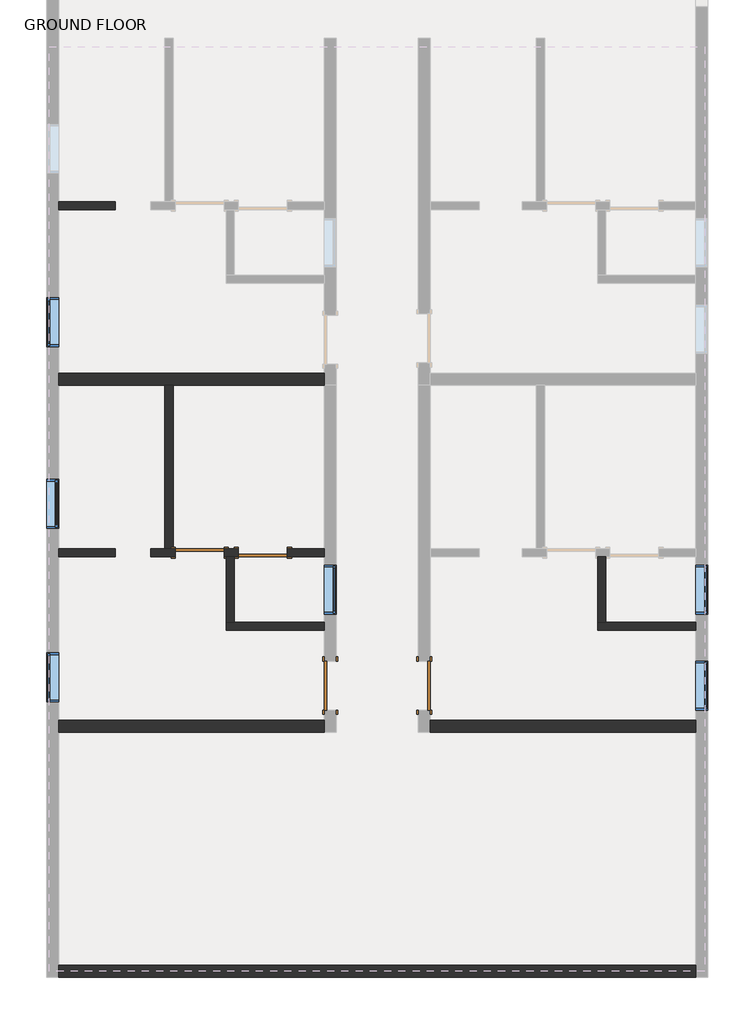
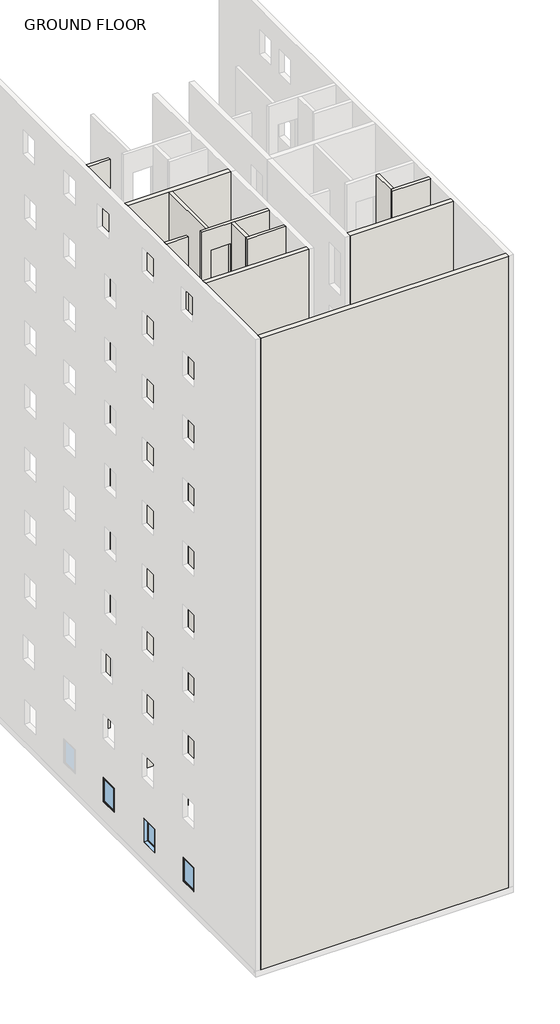
# One storey, part 1 of 7: 12 walls, 6 windows, 4 doors.
"""IFC4 building model written with IfcOpenShell, lengths in millimetres."""

from ifc_helpers import new_model, si_unit, origin, origin_with_axes, place, context, project, spatial, polyline, outline, extrude, faceted_brep, transform, mapped, element, save
from components import door_686f89d2, door_16372e1c, door_a90ba1ad, door_0ca8825f, window_c1f32544

model = new_model("IFC4")

# Units and contexts
model_context = context("Model", 3, world=origin())
ifc_project = project(units=[si_unit("LENGTHUNIT", "METRE", prefix="MILLI")], contexts=[model_context])

# Site, building, storey
site = spatial("IfcSite", under=ifc_project)
building = spatial("IfcBuilding", under=site)
storey = spatial("IfcBuildingStorey", under=building, Name="GROUND FLOOR", Elevation=0.0)

# Doors
placement = place(None, origin())
door_shape = door_686f89d2(model_context)
element("IfcDoor", 1, ObjectType="Single-Flush : 36\" x 84\"", at=placement, inside=storey, context=model_context, shape_type="MappedRepresentation", body=[
    mapped(door_shape, transform((-9863.5902461, -7478.7289408, 0.0), x_axis=(-1.0, 0.0, 0.0), y_axis=(0.0, -1.0, 0.0), z_axis=(0.0, 0.0, 1.0))),
])
door_2_shape = door_16372e1c(model_context)
element("IfcDoor", 2, ObjectType="Single-Flush : 36\" x 84\"", at=placement, inside=storey, context=model_context, shape_type="MappedRepresentation", body=[
    mapped(door_2_shape, transform((-8682.4902461, -7478.7289408, 0.0), x_axis=(-1.0, 0.0, 0.0), y_axis=(0.0, -1.0, 0.0), z_axis=(0.0, 0.0, 1.0))),
])
door_3_shape = door_a90ba1ad(model_context)
element("IfcDoor", 3, ObjectType="Single-Flush : 36\" x 84\"", at=placement, inside=storey, context=model_context, shape_type="MappedRepresentation", body=[
    mapped(door_3_shape, transform((-7425.1902461, -9955.2289408, 0.0), x_axis=(0.0, -1.0, 0.0), y_axis=(1.0, 0.0, 0.0), z_axis=(0.0, 0.0, 1.0))),
])
door_4_shape = door_0ca8825f(model_context)
element("IfcDoor", 4, ObjectType="Single-Flush : 36\" x 84\"", at=placement, inside=storey, context=model_context, shape_type="MappedRepresentation", body=[
    mapped(door_4_shape, transform((-5672.5902461, -9955.2289408, 0.0), x_axis=(0.0, -1.0, 0.0), y_axis=(1.0, 0.0, 0.0), z_axis=(0.0, 0.0, 1.0))),
])

# Walls
element("IfcWall", 5, ObjectType="INNER WALL 2", at=placement, inside=storey, context=model_context, shape_type="Brep", body=[
    faceted_brep([(-605.2902461, -8774.1289408, 0.0), (-2281.6902461, -8774.1289408, 0.0), (-2434.0902461, -8774.1289408, 0.0), (-2434.0902461, -8774.1289408, 32004.0), (-2281.6902461, -8774.1289408, 32004.0), (-605.2902461, -8774.1289408, 32004.0), (-605.2902461, -8926.5289408, 0.0), (-605.2902461, -8926.5289408, 32004.0), (-2434.0902461, -8926.5289408, 32004.0), (-2434.0902461, -8926.5289408, 0.0)], [[[0, 1, 2, 3, 4, 5]], [[6, 7, 8, 9]], [[2, 1, 0, 6, 9]], [[5, 4, 3, 8, 7]], [[3, 2, 9, 8]], [[0, 5, 7, 6]]]),
])
element("IfcWall", 6, ObjectType="INNER WALL 2", at=placement, inside=storey, context=model_context, shape_type="SweptSolid", body=[
    extrude(outline(polyline([(-2281.6902461, -7554.9289408), (-2281.6902461, -8774.1289408), (-2434.0902461, -8774.1289408), (-2434.0902461, -7554.9289408), (-2281.6902461, -7554.9289408)])), origin_with_axes(), (0.0, 0.0, 1.0), 32004.0),
])
element("IfcWall", 7, ObjectType="INNER WALL 2", at=placement, inside=storey, context=model_context, shape_type="Brep", body=[
    faceted_brep([(-9406.3902461, -7554.9289408, 0.0), (-9368.2902461, -7554.9289408, 0.0), (-9215.8902461, -7554.9289408, 0.0), (-9139.6902461, -7554.9289408, 0.0), (-9139.6902461, -7554.9289408, 2133.6), (-8225.2902461, -7554.9289408, 2133.6), (-8225.2902461, -7554.9289408, 0.0), (-7539.4902461, -7554.9289408, 0.0), (-7539.4902461, -7554.9289408, 32004.0), (-9215.8902461, -7554.9289408, 32004.0), (-9368.2902461, -7554.9289408, 32004.0), (-10777.9902461, -7554.9289408, 32004.0), (-10777.9902461, -7554.9289408, 0.0), (-10320.7902461, -7554.9289408, 0.0), (-10320.7902461, -7554.9289408, 2133.6), (-9406.3902461, -7554.9289408, 2133.6), (-9406.3902461, -7554.9289408, 3200.4), (-10320.7902461, -7554.9289408, 3200.4), (-10320.7902461, -7554.9289408, 5334.0), (-9406.3902461, -7554.9289408, 5334.0), (-8225.2902461, -7554.9289408, 3200.4), (-9139.6902461, -7554.9289408, 3200.4), (-9139.6902461, -7554.9289408, 5334.0), (-8225.2902461, -7554.9289408, 5334.0), (-9406.3902461, -7554.9289408, 6400.8), (-10320.7902461, -7554.9289408, 6400.8), (-10320.7902461, -7554.9289408, 8534.4), (-9406.3902461, -7554.9289408, 8534.4), (-8225.2902461, -7554.9289408, 6400.8), (-9139.6902461, -7554.9289408, 6400.8), (-9139.6902461, -7554.9289408, 8534.4), (-8225.2902461, -7554.9289408, 8534.4), (-9406.3902461, -7554.9289408, 9601.2), (-10320.7902461, -7554.9289408, 9601.2), (-10320.7902461, -7554.9289408, 11734.8), (-9406.3902461, -7554.9289408, 11734.8), (-8225.2902461, -7554.9289408, 9601.2), (-9139.6902461, -7554.9289408, 9601.2), (-9139.6902461, -7554.9289408, 11734.8), (-8225.2902461, -7554.9289408, 11734.8), (-9406.3902461, -7554.9289408, 12801.6), (-10320.7902461, -7554.9289408, 12801.6), (-10320.7902461, -7554.9289408, 14935.2), (-9406.3902461, -7554.9289408, 14935.2), (-8225.2902461, -7554.9289408, 12801.6), (-9139.6902461, -7554.9289408, 12801.6), (-9139.6902461, -7554.9289408, 14935.2), (-8225.2902461, -7554.9289408, 14935.2), (-9406.3902461, -7554.9289408, 16002.0), (-10320.7902461, -7554.9289408, 16002.0), (-10320.7902461, -7554.9289408, 18135.6), (-9406.3902461, -7554.9289408, 18135.6), (-8225.2902461, -7554.9289408, 16002.0), (-9139.6902461, -7554.9289408, 16002.0), (-9139.6902461, -7554.9289408, 18135.6), (-8225.2902461, -7554.9289408, 18135.6), (-9406.3902461, -7554.9289408, 19202.4), (-10320.7902461, -7554.9289408, 19202.4), (-10320.7902461, -7554.9289408, 21336.0), (-9406.3902461, -7554.9289408, 21336.0), (-8225.2902461, -7554.9289408, 19202.4), (-9139.6902461, -7554.9289408, 19202.4), (-9139.6902461, -7554.9289408, 21336.0), (-8225.2902461, -7554.9289408, 21336.0), (-9406.3902461, -7554.9289408, 22402.8), (-10320.7902461, -7554.9289408, 22402.8), (-10320.7902461, -7554.9289408, 24536.4), (-9406.3902461, -7554.9289408, 24536.4), (-8225.2902461, -7554.9289408, 22402.8), (-9139.6902461, -7554.9289408, 22402.8), (-9139.6902461, -7554.9289408, 24536.4), (-8225.2902461, -7554.9289408, 24536.4), (-9406.3902461, -7554.9289408, 25603.2), (-10320.7902461, -7554.9289408, 25603.2), (-10320.7902461, -7554.9289408, 27736.8), (-9406.3902461, -7554.9289408, 27736.8), (-8225.2902461, -7554.9289408, 25603.2), (-9139.6902461, -7554.9289408, 25603.2), (-9139.6902461, -7554.9289408, 27736.8), (-8225.2902461, -7554.9289408, 27736.8), (-9406.3902461, -7554.9289408, 28803.6), (-10320.7902461, -7554.9289408, 28803.6), (-10320.7902461, -7554.9289408, 30937.2), (-9406.3902461, -7554.9289408, 30937.2), (-8225.2902461, -7554.9289408, 28803.6), (-9139.6902461, -7554.9289408, 28803.6), (-9139.6902461, -7554.9289408, 30937.2), (-8225.2902461, -7554.9289408, 30937.2), (-9139.6902461, -7402.5289408, 2133.6), (-9139.6902461, -7402.5289408, 0.0), (-9406.3902461, -7402.5289408, 0.0), (-9406.3902461, -7402.5289408, 2133.6), (-10320.7902461, -7402.5289408, 2133.6), (-10320.7902461, -7402.5289408, 0.0), (-10358.8902461, -7402.5289408, 0.0), (-10511.2902461, -7402.5289408, 0.0), (-10777.9902461, -7402.5289408, 0.0), (-10777.9902461, -7402.5289408, 32004.0), (-10511.2902461, -7402.5289408, 32004.0), (-10358.8902461, -7402.5289408, 32004.0), (-7539.4902461, -7402.5289408, 32004.0), (-7539.4902461, -7402.5289408, 0.0), (-8225.2902461, -7402.5289408, 0.0), (-8225.2902461, -7402.5289408, 2133.6), (-9406.3902461, -7402.5289408, 3200.4), (-9406.3902461, -7402.5289408, 5334.0), (-10320.7902461, -7402.5289408, 5334.0), (-10320.7902461, -7402.5289408, 3200.4), (-8225.2902461, -7402.5289408, 3200.4), (-8225.2902461, -7402.5289408, 5334.0), (-9139.6902461, -7402.5289408, 5334.0), (-9139.6902461, -7402.5289408, 3200.4), (-9406.3902461, -7402.5289408, 6400.8), (-9406.3902461, -7402.5289408, 8534.4), (-10320.7902461, -7402.5289408, 8534.4), (-10320.7902461, -7402.5289408, 6400.8), (-8225.2902461, -7402.5289408, 6400.8), (-8225.2902461, -7402.5289408, 8534.4), (-9139.6902461, -7402.5289408, 8534.4), (-9139.6902461, -7402.5289408, 6400.8), (-9406.3902461, -7402.5289408, 9601.2), (-9406.3902461, -7402.5289408, 11734.8), (-10320.7902461, -7402.5289408, 11734.8), (-10320.7902461, -7402.5289408, 9601.2), (-8225.2902461, -7402.5289408, 9601.2), (-8225.2902461, -7402.5289408, 11734.8), (-9139.6902461, -7402.5289408, 11734.8), (-9139.6902461, -7402.5289408, 9601.2), (-9406.3902461, -7402.5289408, 12801.6), (-9406.3902461, -7402.5289408, 14935.2), (-10320.7902461, -7402.5289408, 14935.2), (-10320.7902461, -7402.5289408, 12801.6), (-8225.2902461, -7402.5289408, 12801.6), (-8225.2902461, -7402.5289408, 14935.2), (-9139.6902461, -7402.5289408, 14935.2), (-9139.6902461, -7402.5289408, 12801.6), (-9406.3902461, -7402.5289408, 16002.0), (-9406.3902461, -7402.5289408, 18135.6), (-10320.7902461, -7402.5289408, 18135.6), (-10320.7902461, -7402.5289408, 16002.0), (-8225.2902461, -7402.5289408, 16002.0), (-8225.2902461, -7402.5289408, 18135.6), (-9139.6902461, -7402.5289408, 18135.6), (-9139.6902461, -7402.5289408, 16002.0), (-9406.3902461, -7402.5289408, 19202.4), (-9406.3902461, -7402.5289408, 21336.0), (-10320.7902461, -7402.5289408, 21336.0), (-10320.7902461, -7402.5289408, 19202.4), (-8225.2902461, -7402.5289408, 19202.4), (-8225.2902461, -7402.5289408, 21336.0), (-9139.6902461, -7402.5289408, 21336.0), (-9139.6902461, -7402.5289408, 19202.4), (-9406.3902461, -7402.5289408, 22402.8), (-9406.3902461, -7402.5289408, 24536.4), (-10320.7902461, -7402.5289408, 24536.4), (-10320.7902461, -7402.5289408, 22402.8), (-8225.2902461, -7402.5289408, 22402.8), (-8225.2902461, -7402.5289408, 24536.4), (-9139.6902461, -7402.5289408, 24536.4), (-9139.6902461, -7402.5289408, 22402.8), (-9406.3902461, -7402.5289408, 25603.2), (-9406.3902461, -7402.5289408, 27736.8), (-10320.7902461, -7402.5289408, 27736.8), (-10320.7902461, -7402.5289408, 25603.2), (-8225.2902461, -7402.5289408, 25603.2), (-8225.2902461, -7402.5289408, 27736.8), (-9139.6902461, -7402.5289408, 27736.8), (-9139.6902461, -7402.5289408, 25603.2), (-9406.3902461, -7402.5289408, 28803.6), (-9406.3902461, -7402.5289408, 30937.2), (-10320.7902461, -7402.5289408, 30937.2), (-10320.7902461, -7402.5289408, 28803.6), (-8225.2902461, -7402.5289408, 28803.6), (-8225.2902461, -7402.5289408, 30937.2), (-9139.6902461, -7402.5289408, 30937.2), (-9139.6902461, -7402.5289408, 28803.6)], [[[0, 1, 2, 3, 4, 5, 6, 7, 8, 9, 10, 11, 12, 13, 14, 15], [16, 17, 18, 19], [20, 21, 22, 23], [24, 25, 26, 27], [28, 29, 30, 31], [32, 33, 34, 35], [36, 37, 38, 39], [40, 41, 42, 43], [44, 45, 46, 47], [48, 49, 50, 51], [52, 53, 54, 55], [56, 57, 58, 59], [60, 61, 62, 63], [64, 65, 66, 67], [68, 69, 70, 71], [72, 73, 74, 75], [76, 77, 78, 79], [80, 81, 82, 83], [84, 85, 86, 87]], [[88, 89, 90, 91, 92, 93, 94, 95, 96, 97, 98, 99, 100, 101, 102, 103], [104, 105, 106, 107], [108, 109, 110, 111], [112, 113, 114, 115], [116, 117, 118, 119], [120, 121, 122, 123], [124, 125, 126, 127], [128, 129, 130, 131], [132, 133, 134, 135], [136, 137, 138, 139], [140, 141, 142, 143], [144, 145, 146, 147], [148, 149, 150, 151], [152, 153, 154, 155], [156, 157, 158, 159], [160, 161, 162, 163], [164, 165, 166, 167], [168, 169, 170, 171], [172, 173, 174, 175]], [[96, 95, 94, 93, 13, 12]], [[102, 101, 7, 6]], [[90, 89, 3, 2, 1, 0]], [[11, 10, 9, 8, 100, 99, 98, 97]], [[12, 11, 97, 96]], [[8, 7, 101, 100]], [[14, 13, 93, 92]], [[15, 14, 92, 91]], [[0, 15, 91, 90]], [[4, 3, 89, 88]], [[5, 4, 88, 103]], [[6, 5, 103, 102]], [[17, 16, 104, 107]], [[18, 17, 107, 106]], [[19, 18, 106, 105]], [[16, 19, 105, 104]], [[21, 20, 108, 111]], [[22, 21, 111, 110]], [[23, 22, 110, 109]], [[20, 23, 109, 108]], [[25, 24, 112, 115]], [[26, 25, 115, 114]], [[27, 26, 114, 113]], [[24, 27, 113, 112]], [[29, 28, 116, 119]], [[30, 29, 119, 118]], [[31, 30, 118, 117]], [[28, 31, 117, 116]], [[33, 32, 120, 123]], [[34, 33, 123, 122]], [[35, 34, 122, 121]], [[32, 35, 121, 120]], [[37, 36, 124, 127]], [[38, 37, 127, 126]], [[39, 38, 126, 125]], [[36, 39, 125, 124]], [[41, 40, 128, 131]], [[42, 41, 131, 130]], [[43, 42, 130, 129]], [[40, 43, 129, 128]], [[45, 44, 132, 135]], [[46, 45, 135, 134]], [[47, 46, 134, 133]], [[44, 47, 133, 132]], [[49, 48, 136, 139]], [[50, 49, 139, 138]], [[51, 50, 138, 137]], [[48, 51, 137, 136]], [[53, 52, 140, 143]], [[54, 53, 143, 142]], [[55, 54, 142, 141]], [[52, 55, 141, 140]], [[57, 56, 144, 147]], [[58, 57, 147, 146]], [[59, 58, 146, 145]], [[56, 59, 145, 144]], [[61, 60, 148, 151]], [[62, 61, 151, 150]], [[63, 62, 150, 149]], [[60, 63, 149, 148]], [[65, 64, 152, 155]], [[66, 65, 155, 154]], [[67, 66, 154, 153]], [[64, 67, 153, 152]], [[69, 68, 156, 159]], [[70, 69, 159, 158]], [[71, 70, 158, 157]], [[68, 71, 157, 156]], [[73, 72, 160, 163]], [[74, 73, 163, 162]], [[75, 74, 162, 161]], [[72, 75, 161, 160]], [[77, 76, 164, 167]], [[78, 77, 167, 166]], [[79, 78, 166, 165]], [[76, 79, 165, 164]], [[81, 80, 168, 171]], [[82, 81, 171, 170]], [[83, 82, 170, 169]], [[80, 83, 169, 168]], [[85, 84, 172, 175]], [[86, 85, 175, 174]], [[87, 86, 174, 173]], [[84, 87, 173, 172]]]),
])
element("IfcWall", 8, ObjectType="INNER WALL 2", at=placement, inside=storey, context=model_context, shape_type="SweptSolid", body=[
    extrude(outline(polyline([(-10358.8902461, -4354.5289408), (-10358.8902461, -7402.5289408), (-10511.2902461, -7402.5289408), (-10511.2902461, -4354.5289408), (-10358.8902461, -4354.5289408)])), origin_with_axes(), (0.0, 0.0, 1.0), 32004.0),
])
element("IfcWall", 9, ObjectType="INNER WALL 2", at=placement, inside=storey, context=model_context, shape_type="Brep", body=[
    faceted_brep([(-7539.4902461, -8774.1289408, 0.0), (-9215.8902461, -8774.1289408, 0.0), (-9368.2902461, -8774.1289408, 0.0), (-9368.2902461, -8774.1289408, 32004.0), (-9215.8902461, -8774.1289408, 32004.0), (-7539.4902461, -8774.1289408, 32004.0), (-7539.4902461, -8926.5289408, 0.0), (-7539.4902461, -8926.5289408, 32004.0), (-9368.2902461, -8926.5289408, 32004.0), (-9368.2902461, -8926.5289408, 0.0)], [[[0, 1, 2, 3, 4, 5]], [[6, 7, 8, 9]], [[2, 1, 0, 6, 9]], [[5, 4, 3, 8, 7]], [[0, 5, 7, 6]], [[3, 2, 9, 8]]]),
])
element("IfcWall", 10, ObjectType="INNER WALL 2", at=placement, inside=storey, context=model_context, shape_type="SweptSolid", body=[
    extrude(outline(polyline([(-9215.8902461, -7554.9289408), (-9215.8902461, -8774.1289408), (-9368.2902461, -8774.1289408), (-9368.2902461, -7554.9289408), (-9215.8902461, -7554.9289408)])), origin_with_axes(), (0.0, 0.0, 1.0), 32004.0),
])
element("IfcWall", 11, ObjectType="INNER WALL 2", at=placement, inside=storey, context=model_context, shape_type="SweptSolid", body=[
    extrude(outline(polyline([(-11438.3902461, -1077.9289408), (-12492.4902461, -1077.9289408), (-12492.4902461, -925.5289408), (-11438.3902461, -925.5289408), (-11438.3902461, -1077.9289408)])), origin_with_axes(), (0.0, 0.0, 1.0), 32004.0),
])
element("IfcWall", 12, ObjectType="INNER WALL 2", at=placement, inside=storey, context=model_context, shape_type="SweptSolid", body=[
    extrude(outline(polyline([(-11438.3902461, -7554.9289408), (-12492.4902461, -7554.9289408), (-12492.4902461, -7402.5289408), (-11438.3902461, -7402.5289408), (-11438.3902461, -7554.9289408)])), origin_with_axes(), (0.0, 0.0, 1.0), 32004.0),
])
element("IfcWall", 13, ObjectType="OUTER WALL", at=placement, inside=storey, context=model_context, shape_type="SweptSolid", body=[
    extrude(outline(polyline([(-5558.2902461, -10602.9289408), (-605.2902461, -10602.9289408), (-605.2902461, -10831.5289408), (-5558.2902461, -10831.5289408), (-5558.2902461, -10602.9289408)])), origin_with_axes(), (0.0, 0.0, 1.0), 32004.0),
])
element("IfcWall", 14, ObjectType="OUTER WALL", at=placement, inside=storey, context=model_context, shape_type="Brep", body=[
    faceted_brep([(-7539.4902461, -4125.9289408, 0.0), (-12492.4902461, -4125.9289408, 0.0), (-12492.4902461, -4125.9289408, 32004.0), (-7539.4902461, -4125.9289408, 32004.0), (-7539.4902461, -4354.5289408, 0.0), (-7539.4902461, -4354.5289408, 32004.0), (-10358.8902461, -4354.5289408, 32004.0), (-10511.2902461, -4354.5289408, 32004.0), (-12492.4902461, -4354.5289408, 32004.0), (-12492.4902461, -4354.5289408, 0.0), (-10511.2902461, -4354.5289408, 0.0), (-10358.8902461, -4354.5289408, 0.0)], [[[0, 1, 2, 3]], [[4, 5, 6, 7, 8, 9, 10, 11]], [[1, 0, 4, 11, 10, 9]], [[3, 2, 8, 7, 6, 5]], [[0, 3, 5, 4]], [[2, 1, 9, 8]]]),
])
element("IfcWall", 15, ObjectType="OUTER WALL", at=placement, inside=storey, context=model_context, shape_type="SweptSolid", body=[
    extrude(outline(polyline([(-12492.4902461, -10602.9289408), (-7539.4902461, -10602.9289408), (-7539.4902461, -10831.5289408), (-12492.4902461, -10831.5289408), (-12492.4902461, -10602.9289408)])), origin_with_axes(), (0.0, 0.0, 1.0), 32004.0),
])
element("IfcWall", 16, ObjectType="OUTER WALL", at=placement, inside=storey, context=model_context, shape_type="SweptSolid", body=[
    extrude(outline(polyline([(-605.2902461, -15403.5289408), (-12492.4902461, -15403.5289408), (-12492.4902461, -15174.9289408), (-605.2902461, -15174.9289408), (-605.2902461, -15403.5289408)])), origin_with_axes(), (0.0, 0.0, 1.0), 32004.0),
])

# Windows
window_shape = window_c1f32544(model_context)
element("IfcWindow", 17, ObjectType="Fixed : 36\" x 48\"", at=placement, inside=storey, context=model_context, shape_type="MappedRepresentation", body=[
    mapped(window_shape, transform((-12606.7902461, -3135.3289408, 0.0), x_axis=(0.0, 1.0, 0.0), y_axis=(-1.0, 0.0, 0.0), z_axis=(0.0, 0.0, 1.0))),
])
element("IfcWindow", 18, ObjectType="Fixed : 36\" x 48\"", at=placement, inside=storey, context=model_context, shape_type="MappedRepresentation", body=[
    mapped(window_shape, transform((-12606.7902461, -6602.4289408, 0.0), x_axis=(0.0, -1.0, 0.0), y_axis=(1.0, 0.0, 0.0), z_axis=(0.0, 0.0, 1.0))),
])
element("IfcWindow", 19, ObjectType="Fixed : 36\" x 48\"", at=placement, inside=storey, context=model_context, shape_type="MappedRepresentation", body=[
    mapped(window_shape, transform((-12606.7902461, -9764.7289408, 0.0), x_axis=(0.0, 1.0, 0.0), y_axis=(-1.0, 0.0, 0.0), z_axis=(0.0, 0.0, 1.0))),
])
element("IfcWindow", 20, ObjectType="Fixed : 36\" x 48\"", at=placement, inside=storey, context=model_context, shape_type="MappedRepresentation", body=[
    mapped(window_shape, transform((-490.9902461, -9993.3289408, 0.0), x_axis=(0.0, -1.0, 0.0), y_axis=(1.0, 0.0, 0.0), z_axis=(0.0, 0.0, 1.0))),
])
element("IfcWindow", 21, ObjectType="Fixed : 36\" x 48\"", at=placement, inside=storey, context=model_context, shape_type="MappedRepresentation", body=[
    mapped(window_shape, transform((-490.9902461, -8202.6289408, 0.0), x_axis=(0.0, -1.0, 0.0), y_axis=(1.0, 0.0, 0.0), z_axis=(0.0, 0.0, 1.0))),
])
element("IfcWindow", 22, ObjectType="Fixed : 36\" x 48\"", at=placement, inside=storey, context=model_context, shape_type="MappedRepresentation", body=[
    mapped(window_shape, transform((-7425.1902461, -8202.6289408, 0.0), x_axis=(0.0, -1.0, 0.0), y_axis=(1.0, 0.0, 0.0), z_axis=(0.0, 0.0, 1.0))),
])

save(model, "model.ifc")

# Revit data of these elements
# Type "Single-Flush : 36\" x 84\""
#   Type Mark = "1"
#   Construction Type Id = "MDOOR"
#   Assembly Code = "C1020"
#   Analytic Construction = "Metal"
#   Thickness = 0' - 2"
#   Heat Transfer Coefficient (U) = 0.651978 BTU/(h·ft²·°F)
#   Height = 7' - 0"
#   Trim Projection Ext = 0' - 1"
#   Trim Projection Int = 0' - 1"
#   Trim Width = 0' - 3"
#   Width = 3' - 0"
#   Define Thermal Properties by = 1
#   Door Material = Door - Panel
#   Frame Material = Door - Frame
#   Visual Light Transmittance = 0
#   Solar Heat Gain Coefficient = 0
#   Function = (empty or 0)
#   Wall Closure = (empty or 0)
# Type "INNER WALL 2"
#   Assembly Code = "B2010"
#   Layers, outside or top first: 0' - 6" no material (function 1)
# Type "OUTER WALL"
#   Assembly Code = "B2010"
#   Layers, outside or top first: 0' - 9" no material (function 1)
# Type "Fixed : 36\" x 48\""
#   Type Mark = "1"
#   Construction Type Id = "GSP4R"
#   Assembly Code = "B2020100"
#   Analytic Construction = "1/8 in Pilkington single glazing"
#   Visual Light Transmittance = 0.9
#   Solar Heat Gain Coefficient = 0.78
#   Heat Transfer Coefficient (U) = 0.6496 BTU/(h·ft²·°F)
#   Height = 4' - 0"
#   Default Sill Height = 3' - 0"
#   Width = 3' - 0"
#   Window Inset = 0' - 0 3/4"
#   Define Thermal Properties by = 1
#   Glass Pane Material = Glass
#   Sash Material = Sash
#   Wall Closure = (empty or 0)
# Elements 1, 2, 3, 4 (IfcDoor, "Single-Flush : 36\" x 84\"")
#   Phase Created = New Construction
#   Materials on its faces: "Door - Frame", "Door - Panel"
# Elements 5, 6, 7, 8, 9, 10, 11, 12 (IfcWall, "INNER WALL 2")
#   Top Offset = 0' - 0"
#   Base Offset = 0' - 0"
#   Unconnected Height = 105' - 0"
#   wall height = 105' - 0"
#   Phase Created = New Construction
#   Base Constraint = GROUND FLOOR
#   Materials on its faces: "Default Wall"
# Elements 13, 14, 15, 16 (IfcWall, "OUTER WALL")
#   Top Offset = 0' - 0"
#   Base Offset = 0' - 0"
#   Unconnected Height = 105' - 0"
#   wall height = 105' - 0"
#   Phase Created = New Construction
#   Base Constraint = GROUND FLOOR
#   Materials on its faces: "Default Wall"
# Element 17 (IfcWindow, "Fixed : 36\" x 48\"")
#   Mark = "8"
#   Phase Created = New Construction
#   Materials on its faces: "Sash", "Glass"
# Element 18 (IfcWindow, "Fixed : 36\" x 48\"")
#   Mark = "9"
#   Phase Created = New Construction
#   Materials on its faces: "Sash", "Glass"
# Element 19 (IfcWindow, "Fixed : 36\" x 48\"")
#   Mark = "10"
#   Phase Created = New Construction
#   Materials on its faces: "Sash", "Glass"
# Element 20 (IfcWindow, "Fixed : 36\" x 48\"")
#   Mark = "11"
#   Phase Created = New Construction
#   Materials on its faces: "Sash", "Glass"
# Element 21 (IfcWindow, "Fixed : 36\" x 48\"")
#   Mark = "12"
#   Phase Created = New Construction
#   Materials on its faces: "Sash", "Glass"
# Element 22 (IfcWindow, "Fixed : 36\" x 48\"")
#   Mark = "23"
#   Phase Created = New Construction
#   Materials on its faces: "Sash", "Glass"
# Materials
#   "Door - Panel": class "Wood", colour RGB 210 159 95, transparency 0
#   "Door - Frame": colour RGB 118 70 51, transparency 0
#   "Glass": class "Glass", colour RGB 0 128 192, transparency 0.75, Description = "Soda Lime Glass", Cost = 0
#   "Sash": class "Wood", colour RGB 224 178 126, transparency 0
#   "Default Wall": colour RGB 128 128 128, transparency 0
